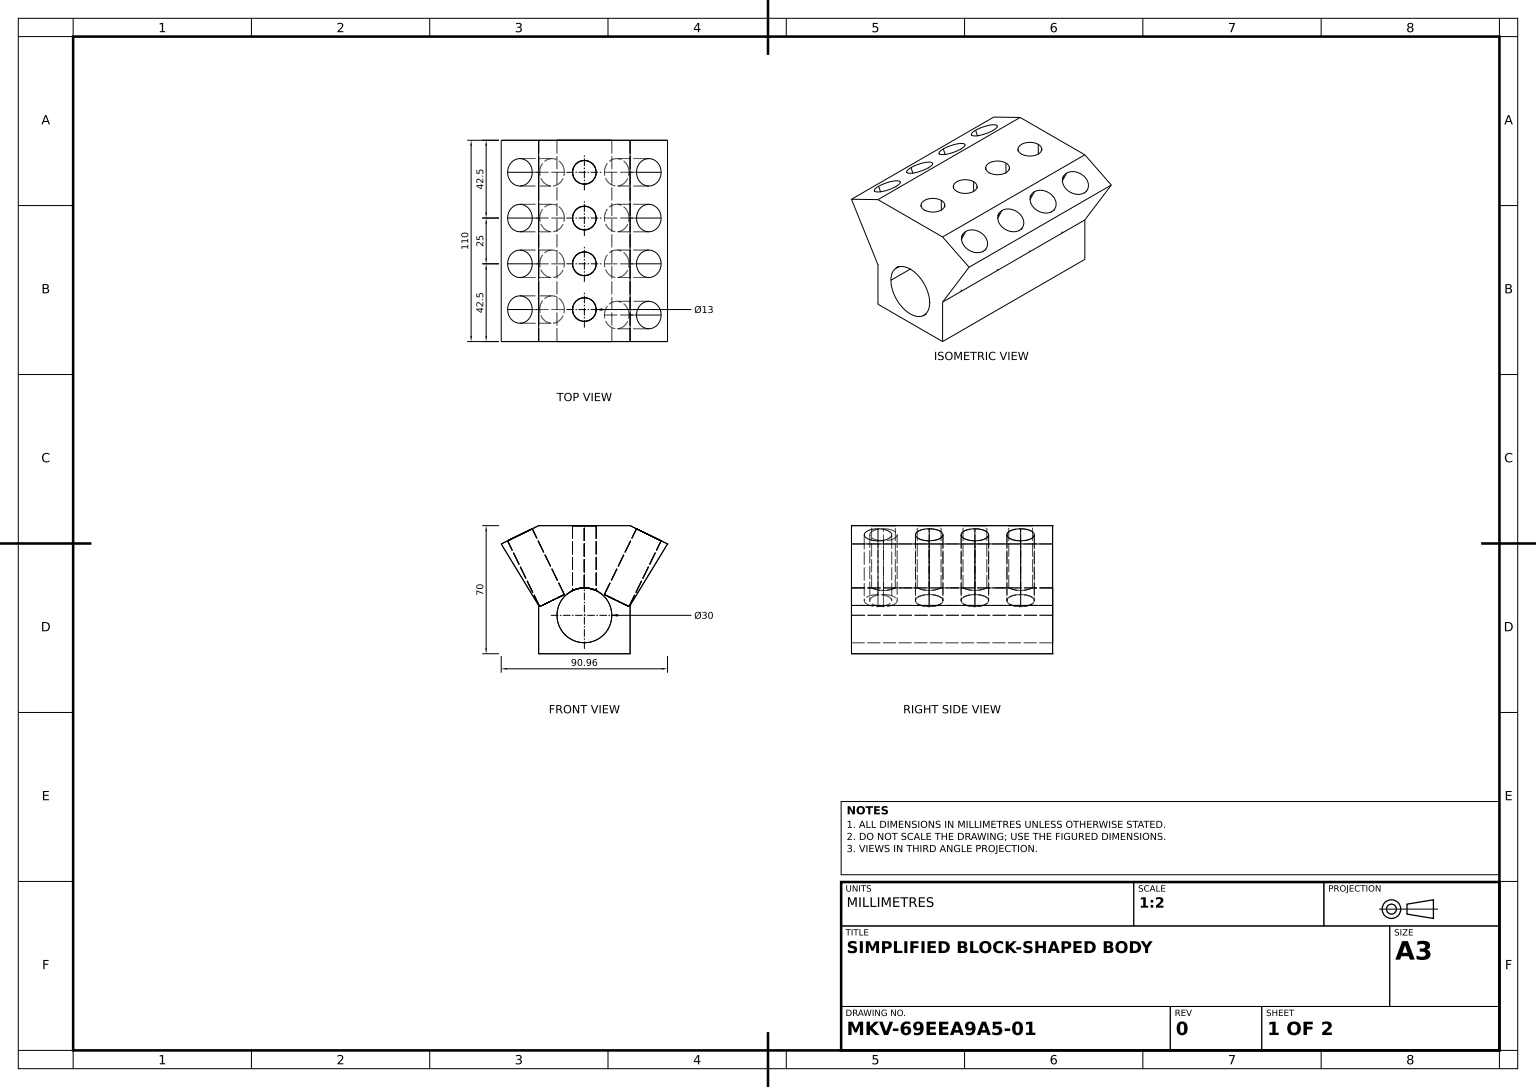
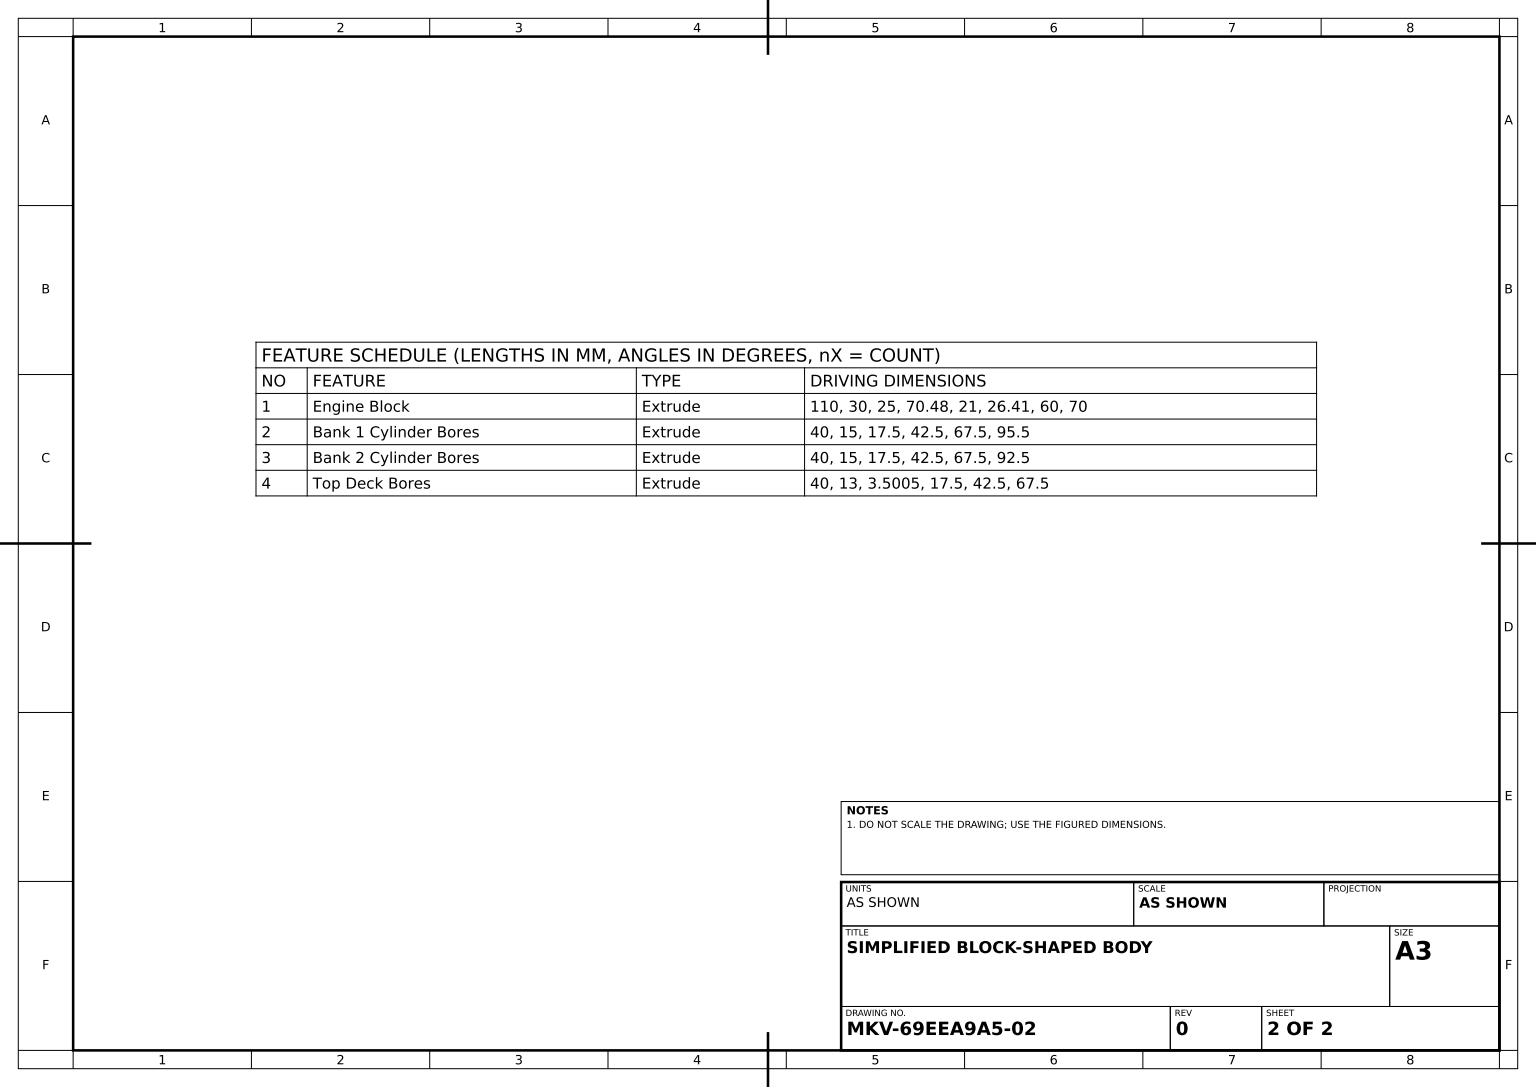
SolidWorks part; units mm, degrees
material "Plain Carbon Steel"
ref_plane "Front Plane" through (0, 0, 0) normal (0, 0, 1) x (1, 0, 0)
ref_plane "Top Plane" through (0, 0, 0) normal (0, 1, 0) x (1, 0, 0)
ref_plane "Right Plane" through (0, 0, 0) normal (1, 0, 0) x (0, 0, -1)
sketch "Block Profile Sketch" plane through (0, 0, 0) normal (0, 0, 1) x (1, 0, 0)
  line L0 (0, 0) -> (25, 0)
  line L1 (25, 0) -> (-25, 0)
  line L2 (25, 0) -> (25, 26.41)
  line L3 (-25, 0) -> (-25, 26.41)
  line L8 (0, 0) -> (25, 0)
  line L9 (0, 70) -> (-25, 70)
  line L11 (0, 0) -> (-25, 0)
  line L12 (45.48, 60) -> (25, 26.41)
  line L14 (-25, 70) -> (25, 70)
  line L15 (-45.48, 60) -> (-25, 26.41)
  line L16 (-45.48, 60) -> (-25, 70)
  line L17 (25, 70) -> (45.48, 60)
  circle A0 centre (0, 21) radius 15
  dimension "D1" = 25
  dimension "D2" = 30
  dimension "D3" = 70.48
  dimension "D4" = 21
  dimension "D5" = 26.41
  dimension "D6" = 60
  dimension "D7" = 70
extrude "Engine Block" add sketch "Block Profile Sketch" against normal blind 110 contours L17 L14 L9 L16 L15 L3 L1 L0 L2 L12 A0
sketch "Bank 1 Bores Sketch" plane through (32.4124, 66.3807, 0) normal (0.4388, 0.8986, 0) x (0.8986, -0.4388, 0)
  line L0 (3.1466, 0) -> (3.1466, 110)
  line L1 (-8.2489, 0) -> (14.5422, 0) construction
  line L2 (-8.2489, 110) -> (14.5422, 110) construction
  line L4 (14.5422, 110) -> (14.5422, 0) construction
  line L5 (14.5422, 14.5) -> (3.1466, 14.5)
  line L7 (14.5422, 42.5) -> (3.1466, 42.5)
  line L9 (14.5422, 67.5) -> (3.1466, 67.5)
  line L11 (14.5422, 92.5) -> (3.1466, 92.5)
  circle A0 centre (3.1466, 14.5) radius 7.5
  circle A1 centre (3.1466, 42.5) radius 7.5
  circle A2 centre (3.1466, 67.5) radius 7.5
  circle A3 centre (3.1466, 92.5) radius 7.5
  dimension "D1" = 15
  dimension "D2" = 15
  dimension "D3" = 15
  dimension "D4" = 15
  dimension "D5" = 15
  dimension "D6" = 17.5
  dimension "D7" = 42.5
  dimension "D8" = 67.5
  dimension "D9" = 95.5
extrude "Bank 1 Cylinder Bores" cut sketch "Bank 1 Bores Sketch" against normal blind 40 contours L0 A3 | L0 A3 L11 | L11 A3 L0 | L0 A2 L9 | L9 A2 L0 | L0 A2 | L0 A1 | L7 A1 L0 | L0 A1 L7 | L0 A0 | L5 A0 L0 | L0 A0 L5
sketch "Bank 2 Bores Sketch" plane through (-32.4124, 66.3807, 0) normal (-0.4388, 0.8986, 0) x (0.8986, 0.4388, 0)
  line L0 (-3.1466, 0) -> (-3.1466, 17.5)
  line L1 (-14.5422, 0) -> (8.2489, 0) construction
  line L2 (-3.1466, 0) -> (-3.1466, 42.5)
  line L3 (-3.1466, 42.5) -> (-3.1466, 0)
  line L4 (-3.1466, 0) -> (-3.1466, 67.5)
  line L5 (-3.1466, 67.5) -> (-3.1466, 0)
  line L6 (-3.1466, 0) -> (-3.1466, 92.5)
  circle A0 centre (-3.1466, 92.5) radius 7.5
  circle A1 centre (-3.1466, 67.5) radius 7.5
  circle A2 centre (-3.1466, 42.5) radius 7.5
  circle A3 centre (-3.1466, 17.5) radius 7.5
  dimension "D1" = 15
  dimension "D2" = 15
  dimension "D3" = 15
  dimension "D4" = 7.5
  dimension "D5" = 15
  dimension "D6" = 17.5
  dimension "D7" = 42.5
  dimension "D8" = 67.5
  dimension "D9" = 92.5
extrude "Bank 2 Cylinder Bores" cut sketch "Bank 2 Bores Sketch" against normal blind 40
sketch "Top Deck Bores Sketch" plane through (0, 70, 0) normal (0, 1, 0) x (1, 0, 0)
  line L0 (0, 110) -> (0, 0)
  line L1 (-25, 110) -> (25, 110) construction
  line L2 (-28.5005, 92.5) -> (28.5005, 92.5)
  line L3 (0, 110) -> (0, 67.5)
  line L4 (0, 67.5) -> (0, 110)
  line L5 (0, 110) -> (0, 17.5)
  line L6 (0, 17.5) -> (0, 110)
  line L7 (0, 110) -> (0, 42.5)
  line L8 (0, 42.5) -> (0, 110)
  line L9 (25, 110) -> (25, 0) construction
  line L10 (-25, 0) -> (25, 0) construction
  circle A0 centre (0, 92.5) radius 6.5
  circle A1 centre (0, 67.5) radius 6.5
  circle A2 centre (0, 42.5) radius 6.5
  circle A3 centre (0, 17.5) radius 6.5
  ellipse E0 centre (-35.24, 92.5) end of major axis (-35.24, 100) minor radius 6.7395 construction
  ellipse E1 centre (35.24, 92.5) end of major axis (35.24, 85) minor radius 6.7395 construction
  dimension "D1" = 13
  dimension "D2" = 13
  dimension "D3" = 13
  dimension "D4" = 13
  dimension "D5" = 13
  dimension "D6" = 3.5005
  dimension "D7" = 17.5
  dimension "D8" = 42.5
  dimension "D9" = 67.5
extrude "Top Deck Bores" cut sketch "Top Deck Bores Sketch" against normal blind 40
